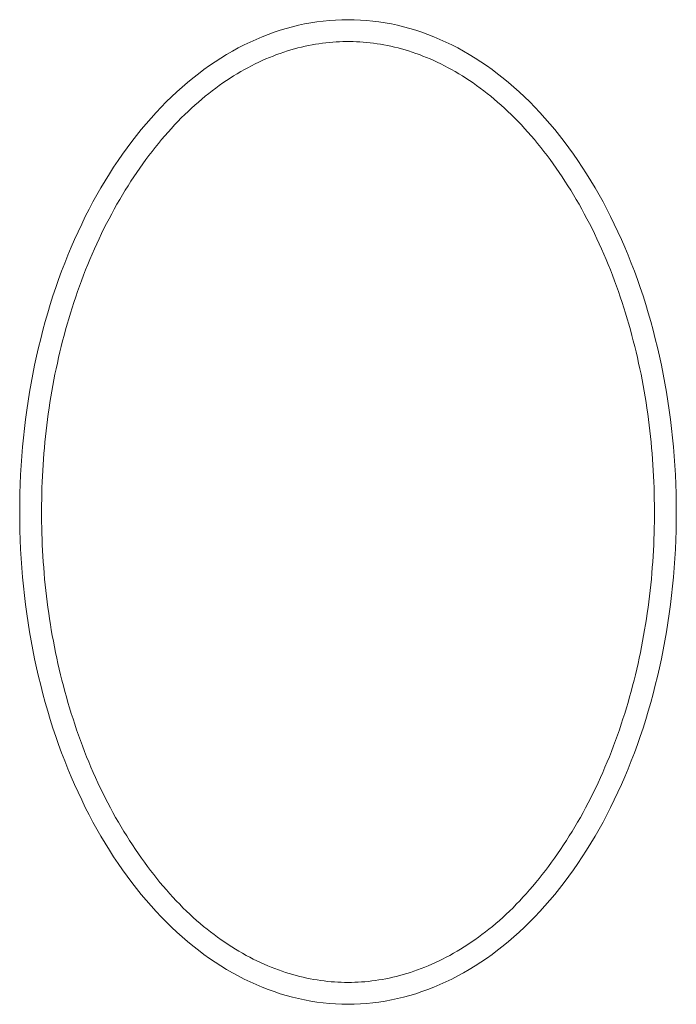
# Model space of a CAD drawing. Units: inches. Extents: x 963 to 2075, y 289 to 2657.
# Tile 52 of 98: x 1538 to 1555, y 1765 to 1790. Entities that reach past the tile are written whole.
import ezdxf

# ---------------------------------------------------------------- set-up
doc = ezdxf.new("R2010")
doc.units = ezdxf.units.IN
doc.layers.add('A-FURN', color=8, linetype='Continuous', lineweight=18)

# ---------------------------------------------------------------- blocks, each defined once
blk = doc.blocks.new('TABLE-OVAL')
at = {"ltscale": 0.03}
blk.add_polyline3d([(7.656, -0.197, 0), (7.809, -0.194, 0), (7.963, -0.188, 0), (8.116, -0.177, 0), (8.269, -0.162, 0), (8.422, -0.142, 0), (8.575, -0.118, 0), (8.727, -0.09, 0), (8.879, -0.057, 0), (9.031, -0.021, 0), (9.182, 0.021, 0), (9.332, 0.066, 0), (9.482, 0.116, 0), (9.632, 0.17, 0), (9.78, 0.228, 0), (9.928, 0.29, 0), (10.075, 0.357, 0), (10.221, 0.428, 0), (10.366, 0.503, 0), (10.51, 0.582, 0), (10.653, 0.665, 0), (10.796, 0.752, 0), (10.937, 0.843, 0), (11.076, 0.938, 0), (11.215, 1.037, 0), (11.352, 1.14, 0), (11.488, 1.247, 0), (11.623, 1.358, 0), (11.756, 1.472, 0), (11.888, 1.59, 0), (12.018, 1.712, 0), (12.147, 1.838, 0), (12.274, 1.967, 0), (12.399, 2.1, 0), (12.523, 2.237, 0), (12.645, 2.376, 0), (12.765, 2.52, 0), (12.883, 2.666, 0), (13, 2.817, 0), (13.114, 2.97, 0), (13.227, 3.126, 0), (13.337, 3.286, 0), (13.446, 3.449, 0), (13.552, 3.615, 0), (13.657, 3.784, 0), (13.759, 3.955, 0), (13.859, 4.13, 0), (13.957, 4.308, 0), (14.052, 4.488, 0), (14.145, 4.671, 0), (14.236, 4.856, 0), (14.325, 5.044, 0), (14.411, 5.235, 0), (14.495, 5.428, 0), (14.576, 5.623, 0), (14.655, 5.821, 0), (14.731, 6.021, 0), (14.805, 6.222, 0), (14.877, 6.426, 0), (14.945, 6.632, 0), (15.011, 6.84, 0), (15.075, 7.05, 0), (15.135, 7.261, 0), (15.193, 7.475, 0), (15.249, 7.689, 0), (15.301, 7.906, 0), (15.351, 8.123, 0), (15.399, 8.343, 0), (15.443, 8.563, 0), (15.485, 8.785, 0), (15.523, 9.007, 0), (15.559, 9.231, 0), (15.592, 9.456, 0), (15.623, 9.682, 0), (15.65, 9.908, 0), (15.675, 10.136, 0), (15.697, 10.364, 0), (15.715, 10.592, 0), (15.731, 10.821, 0), (15.744, 11.051, 0), (15.755, 11.28, 0), (15.762, 11.51, 0), (15.766, 11.741, 0), (15.768, 11.971, 0), (15.766, 12.201, 0), (15.762, 12.431, 0), (15.755, 12.661, 0), (15.744, 12.891, 0), (15.731, 13.12, 0), (15.715, 13.349, 0), (15.697, 13.578, 0), (15.675, 13.806, 0), (15.65, 14.033, 0), (15.623, 14.26, 0), (15.592, 14.486, 0), (15.559, 14.71, 0), (15.523, 14.934, 0), (15.485, 15.157, 0), (15.443, 15.379, 0), (15.399, 15.599, 0), (15.351, 15.818, 0), (15.301, 16.036, 0), (15.249, 16.252, 0), (15.193, 16.467, 0), (15.135, 16.68, 0), (15.075, 16.892, 0), (15.011, 17.101, 0), (14.945, 17.309, 0), (14.877, 17.515, 0), (14.805, 17.719, 0), (14.731, 17.921, 0), (14.655, 18.121, 0), (14.576, 18.318, 0), (14.495, 18.514, 0), (14.411, 18.707, 0), (14.325, 18.897, 0), (14.236, 19.085, 0), (14.145, 19.271, 0), (14.052, 19.454, 0), (13.957, 19.634, 0), (13.859, 19.811, 0), (13.759, 19.986, 0), (13.657, 20.158, 0), (13.552, 20.327, 0), (13.446, 20.493, 0), (13.337, 20.656, 0), (13.227, 20.815, 0), (13.114, 20.972, 0), (13, 21.125, 0), (12.883, 21.275, 0), (12.765, 21.422, 0), (12.645, 21.565, 0), (12.523, 21.705, 0), (12.399, 21.842, 0), (12.274, 21.974, 0), (12.147, 22.104, 0), (12.018, 22.229, 0), (11.888, 22.351, 0), (11.756, 22.47, 0), (11.623, 22.584, 0), (11.488, 22.695, 0), (11.352, 22.802, 0), (11.215, 22.905, 0), (11.076, 23.004, 0), (10.937, 23.099, 0), (10.796, 23.19, 0), (10.653, 23.277, 0), (10.51, 23.36, 0), (10.366, 23.439, 0), (10.221, 23.514, 0), (10.075, 23.585, 0), (9.928, 23.651, 0), (9.78, 23.714, 0), (9.632, 23.772, 0), (9.482, 23.826, 0), (9.332, 23.876, 0), (9.182, 23.921, 0), (9.031, 23.962, 0), (8.879, 23.999, 0), (8.727, 24.032, 0), (8.575, 24.06, 0), (8.422, 24.084, 0), (8.269, 24.103, 0), (8.116, 24.119, 0), (7.963, 24.13, 0), (7.809, 24.136, 0), (7.656, 24.138, 0), (7.502, 24.136, 0), (7.349, 24.13, 0), (7.196, 24.119, 0), (7.042, 24.103, 0), (6.89, 24.084, 0), (6.737, 24.06, 0), (6.585, 24.032, 0), (6.433, 23.999, 0), (6.281, 23.962, 0), (6.13, 23.921, 0), (5.979, 23.876, 0), (5.83, 23.826, 0), (5.68, 23.772, 0), (5.532, 23.714, 0), (5.384, 23.651, 0), (5.237, 23.585, 0), (5.091, 23.514, 0), (4.946, 23.439, 0), (4.802, 23.36, 0), (4.658, 23.277, 0), (4.516, 23.19, 0), (4.375, 23.099, 0), (4.236, 23.004, 0), (4.097, 22.905, 0), (3.96, 22.802, 0), (3.824, 22.695, 0), (3.689, 22.584, 0), (3.556, 22.47, 0), (3.424, 22.351, 0), (3.294, 22.229, 0), (3.165, 22.104, 0), (3.038, 21.974, 0), (2.913, 21.842, 0), (2.789, 21.705, 0), (2.667, 21.565, 0), (2.547, 21.422, 0), (2.429, 21.275, 0), (2.312, 21.125, 0), (2.198, 20.972, 0), (2.085, 20.815, 0), (1.975, 20.656, 0), (1.866, 20.493, 0), (1.76, 20.327, 0), (1.655, 20.158, 0), (1.553, 19.986, 0), (1.453, 19.811, 0), (1.355, 19.634, 0), (1.26, 19.454, 0), (1.166, 19.271, 0), (1.076, 19.085, 0), (0.987, 18.897, 0), (0.901, 18.707, 0), (0.817, 18.514, 0), (0.736, 18.318, 0), (0.657, 18.121, 0), (0.58, 17.921, 0), (0.507, 17.719, 0), (0.435, 17.515, 0), (0.367, 17.309, 0), (0.301, 17.101, 0), (0.237, 16.892, 0), (0.177, 16.68, 0), (0.118, 16.467, 0), (0.063, 16.252, 0), (0.01, 16.036, 0), (-0.039, 15.818, 0), (-0.087, 15.599, 0), (-0.131, 15.379, 0), (-0.173, 15.157, 0), (-0.211, 14.934, 0), (-0.247, 14.71, 0), (-0.281, 14.486, 0), (-0.311, 14.26, 0), (-0.338, 14.033, 0), (-0.363, 13.806, 0), (-0.385, 13.578, 0), (-0.403, 13.349, 0), (-0.419, 13.12, 0), (-0.432, 12.891, 0), (-0.443, 12.661, 0), (-0.45, 12.431, 0), (-0.454, 12.201, 0), (-0.456, 11.971, 0), (-0.454, 11.741, 0), (-0.45, 11.51, 0), (-0.443, 11.28, 0), (-0.432, 11.051, 0), (-0.419, 10.821, 0), (-0.403, 10.592, 0), (-0.385, 10.364, 0), (-0.363, 10.136, 0), (-0.338, 9.908, 0), (-0.311, 9.682, 0), (-0.281, 9.456, 0), (-0.247, 9.231, 0), (-0.211, 9.007, 0), (-0.173, 8.785, 0), (-0.131, 8.563, 0), (-0.087, 8.343, 0), (-0.039, 8.123, 0), (0.01, 7.906, 0), (0.063, 7.689, 0), (0.118, 7.475, 0), (0.177, 7.261, 0), (0.237, 7.05, 0), (0.301, 6.84, 0), (0.367, 6.632, 0), (0.435, 6.426, 0), (0.507, 6.222, 0), (0.58, 6.021, 0), (0.657, 5.821, 0), (0.736, 5.623, 0), (0.817, 5.428, 0), (0.901, 5.235, 0), (0.987, 5.044, 0), (1.076, 4.856, 0), (1.166, 4.671, 0), (1.26, 4.488, 0), (1.355, 4.308, 0), (1.453, 4.13, 0), (1.553, 3.955, 0), (1.655, 3.784, 0), (1.76, 3.615, 0), (1.866, 3.449, 0), (1.975, 3.286, 0), (2.085, 3.126, 0), (2.198, 2.97, 0), (2.312, 2.817, 0), (2.429, 2.666, 0), (2.547, 2.52, 0), (2.667, 2.376, 0), (2.789, 2.237, 0), (2.913, 2.1, 0), (3.038, 1.967, 0), (3.165, 1.838, 0), (3.294, 1.712, 0), (3.424, 1.59, 0), (3.556, 1.472, 0), (3.689, 1.358, 0), (3.824, 1.247, 0), (3.96, 1.14, 0), (4.097, 1.037, 0), (4.236, 0.938, 0), (4.375, 0.843, 0), (4.516, 0.752, 0), (4.658, 0.665, 0), (4.802, 0.582, 0), (4.946, 0.503, 0), (5.091, 0.428, 0), (5.237, 0.357, 0), (5.384, 0.29, 0), (5.532, 0.228, 0), (5.68, 0.17, 0), (5.83, 0.116, 0), (5.979, 0.066, 0), (6.13, 0.021, 0), (6.281, -0.021, 0), (6.433, -0.057, 0), (6.585, -0.09, 0), (6.737, -0.118, 0), (6.89, -0.142, 0), (7.042, -0.162, 0), (7.196, -0.177, 0), (7.349, -0.188, 0), (7.502, -0.194, 0), (7.656, -0.197, 0)], dxfattribs=at)
blk.add_polyline3d([(7.656, 0.344, 0), (7.739, 0.345, 0), (7.822, 0.347, 0), (7.906, 0.351, 0), (7.99, 0.356, 0), (8.074, 0.362, 0), (8.159, 0.37, 0), (8.244, 0.38, 0), (8.33, 0.391, 0), (8.415, 0.404, 0), (8.501, 0.418, 0), (8.588, 0.434, 0), (8.674, 0.451, 0), (8.761, 0.47, 0), (8.848, 0.491, 0), (8.935, 0.513, 0), (9.023, 0.538, 0), (9.11, 0.563, 0), (9.198, 0.591, 0), (9.286, 0.62, 0), (9.375, 0.651, 0), (9.463, 0.684, 0), (9.552, 0.719, 0), (9.64, 0.755, 0), (9.729, 0.794, 0), (9.818, 0.834, 0), (9.907, 0.876, 0), (9.995, 0.92, 0), (10.084, 0.966, 0), (10.173, 1.013, 0), (10.262, 1.063, 0), (10.35, 1.114, 0), (10.439, 1.167, 0), (10.527, 1.222, 0), (10.615, 1.279, 0), (10.703, 1.338, 0), (10.791, 1.398, 0), (10.878, 1.461, 0), (10.965, 1.525, 0), (11.052, 1.592, 0), (11.139, 1.66, 0), (11.225, 1.73, 0), (11.311, 1.802, 0), (11.396, 1.876, 0), (11.481, 1.952, 0), (11.565, 2.03, 0), (11.649, 2.109, 0), (11.733, 2.191, 0), (11.815, 2.275, 0), (11.898, 2.361, 0), (11.98, 2.448, 0), (12.061, 2.537, 0), (12.141, 2.629, 0), (12.221, 2.721, 0), (12.301, 2.816, 0), (12.379, 2.912, 0), (12.457, 3.01, 0), (12.535, 3.11, 0), (12.611, 3.211, 0), (12.687, 3.314, 0), (12.762, 3.418, 0), (12.836, 3.524, 0), (12.909, 3.632, 0), (12.982, 3.741, 0), (13.053, 3.851, 0), (13.124, 3.963, 0), (13.194, 4.076, 0), (13.262, 4.191, 0), (13.33, 4.307, 0), (13.397, 4.424, 0), (13.463, 4.543, 0), (13.528, 4.662, 0), (13.591, 4.783, 0), (13.654, 4.906, 0), (13.716, 5.029, 0), (13.776, 5.154, 0), (13.835, 5.279, 0), (13.893, 5.406, 0), (13.95, 5.534, 0), (14.006, 5.663, 0), (14.061, 5.792, 0), (14.114, 5.923, 0), (14.166, 6.055, 0), (14.217, 6.188, 0), (14.266, 6.321, 0), (14.314, 6.455, 0), (14.361, 6.589, 0), (14.406, 6.723, 0), (14.45, 6.858, 0), (14.493, 6.993, 0), (14.535, 7.129, 0), (14.575, 7.265, 0), (14.614, 7.401, 0), (14.652, 7.537, 0), (14.688, 7.674, 0), (14.724, 7.811, 0), (14.758, 7.948, 0), (14.791, 8.086, 0), (14.822, 8.223, 0), (14.852, 8.361, 0), (14.882, 8.5, 0), (14.909, 8.638, 0), (14.936, 8.777, 0), (14.961, 8.916, 0), (14.986, 9.055, 0), (15.009, 9.194, 0), (15.031, 9.334, 0), (15.051, 9.473, 0), (15.071, 9.613, 0), (15.089, 9.753, 0), (15.106, 9.893, 0), (15.122, 10.033, 0), (15.137, 10.174, 0), (15.151, 10.314, 0), (15.163, 10.455, 0), (15.175, 10.596, 0), (15.185, 10.736, 0), (15.194, 10.877, 0), (15.202, 11.018, 0), (15.209, 11.159, 0), (15.215, 11.3, 0), (15.219, 11.441, 0), (15.223, 11.583, 0), (15.225, 11.724, 0), (15.227, 11.865, 0), (15.227, 12.006, 0), (15.226, 12.147, 0), (15.224, 12.288, 0), (15.221, 12.43, 0), (15.217, 12.571, 0), (15.212, 12.712, 0), (15.205, 12.853, 0), (15.198, 12.994, 0), (15.19, 13.135, 0), (15.18, 13.276, 0), (15.169, 13.416, 0), (15.157, 13.557, 0), (15.144, 13.698, 0), (15.13, 13.838, 0), (15.114, 13.978, 0), (15.098, 14.119, 0), (15.08, 14.259, 0), (15.061, 14.399, 0), (15.041, 14.538, 0), (15.02, 14.678, 0), (14.997, 14.817, 0), (14.974, 14.956, 0), (14.949, 15.095, 0), (14.923, 15.234, 0), (14.896, 15.373, 0), (14.867, 15.511, 0), (14.837, 15.649, 0), (14.806, 15.787, 0), (14.774, 15.925, 0), (14.741, 16.062, 0), (14.706, 16.199, 0), (14.67, 16.336, 0), (14.633, 16.473, 0), (14.595, 16.609, 0), (14.555, 16.745, 0), (14.514, 16.881, 0), (14.472, 17.016, 0), (14.428, 17.151, 0), (14.384, 17.286, 0), (14.338, 17.42, 0), (14.29, 17.554, 0), (14.241, 17.687, 0), (14.191, 17.821, 0), (14.14, 17.953, 0), (14.087, 18.084, 0), (14.034, 18.214, 0), (13.978, 18.344, 0), (13.922, 18.472, 0), (13.865, 18.599, 0), (13.806, 18.725, 0), (13.746, 18.85, 0), (13.685, 18.974, 0), (13.623, 19.097, 0), (13.56, 19.219, 0), (13.495, 19.339, 0), (13.43, 19.458, 0), (13.364, 19.576, 0), (13.296, 19.693, 0), (13.228, 19.808, 0), (13.159, 19.922, 0), (13.089, 20.035, 0), (13.017, 20.146, 0), (12.945, 20.255, 0), (12.873, 20.364, 0), (12.799, 20.47, 0), (12.724, 20.576, 0), (12.649, 20.679, 0), (12.573, 20.781, 0), (12.496, 20.882, 0), (12.418, 20.981, 0), (12.34, 21.078, 0), (12.261, 21.173, 0), (12.182, 21.267, 0), (12.101, 21.359, 0), (12.02, 21.449, 0), (11.939, 21.537, 0), (11.857, 21.624, 0), (11.774, 21.709, 0), (11.691, 21.791, 0), (11.607, 21.872, 0), (11.523, 21.951, 0), (11.438, 22.028, 0), (11.353, 22.103, 0), (11.268, 22.176, 0), (11.182, 22.247, 0), (11.095, 22.316, 0), (11.009, 22.383, 0), (10.922, 22.449, 0), (10.835, 22.512, 0), (10.747, 22.574, 0), (10.659, 22.633, 0), (10.571, 22.691, 0), (10.483, 22.747, 0), (10.395, 22.801, 0), (10.306, 22.854, 0), (10.217, 22.904, 0), (10.129, 22.952, 0), (10.04, 22.999, 0), (9.951, 23.044, 0), (9.862, 23.087, 0), (9.773, 23.128, 0), (9.685, 23.167, 0), (9.596, 23.205, 0), (9.507, 23.24, 0), (9.419, 23.274, 0), (9.331, 23.306, 0), (9.242, 23.336, 0), (9.154, 23.365, 0), (9.067, 23.391, 0), (8.979, 23.416, 0), (8.892, 23.44, 0), (8.804, 23.461, 0), (8.718, 23.481, 0), (8.631, 23.499, 0), (8.544, 23.516, 0), (8.458, 23.531, 0), (8.373, 23.545, 0), (8.287, 23.557, 0), (8.202, 23.567, 0), (8.117, 23.576, 0), (8.032, 23.583, 0), (7.948, 23.589, 0), (7.864, 23.593, 0), (7.781, 23.596, 0), (7.697, 23.597, 0), (7.615, 23.597, 0), (7.531, 23.596, 0), (7.448, 23.593, 0), (7.364, 23.589, 0), (7.28, 23.583, 0), (7.195, 23.576, 0), (7.11, 23.567, 0), (7.025, 23.557, 0), (6.939, 23.545, 0), (6.854, 23.531, 0), (6.767, 23.516, 0), (6.681, 23.499, 0), (6.594, 23.481, 0), (6.507, 23.461, 0), (6.42, 23.44, 0), (6.333, 23.416, 0), (6.245, 23.391, 0), (6.158, 23.365, 0), (6.07, 23.336, 0), (5.981, 23.306, 0), (5.893, 23.274, 0), (5.805, 23.24, 0), (5.716, 23.205, 0), (5.627, 23.167, 0), (5.539, 23.128, 0), (5.45, 23.087, 0), (5.361, 23.044, 0), (5.272, 22.999, 0), (5.183, 22.952, 0), (5.095, 22.904, 0), (5.006, 22.854, 0), (4.917, 22.801, 0), (4.829, 22.747, 0), (4.741, 22.691, 0), (4.653, 22.633, 0), (4.565, 22.574, 0), (4.477, 22.512, 0), (4.39, 22.449, 0), (4.303, 22.383, 0), (4.216, 22.316, 0), (4.13, 22.247, 0), (4.044, 22.176, 0), (3.959, 22.103, 0), (3.874, 22.028, 0), (3.789, 21.951, 0), (3.705, 21.872, 0), (3.621, 21.791, 0), (3.538, 21.709, 0), (3.455, 21.624, 0), (3.373, 21.537, 0), (3.292, 21.449, 0), (3.211, 21.359, 0), (3.13, 21.267, 0), (3.051, 21.173, 0), (2.972, 21.078, 0), (2.893, 20.981, 0), (2.816, 20.882, 0), (2.739, 20.781, 0), (2.663, 20.679, 0), (2.588, 20.576, 0), (2.513, 20.47, 0), (2.439, 20.364, 0), (2.366, 20.255, 0), (2.294, 20.146, 0), (2.223, 20.035, 0), (2.153, 19.922, 0), (2.084, 19.808, 0), (2.016, 19.693, 0), (1.948, 19.576, 0), (1.882, 19.458, 0), (1.817, 19.339, 0), (1.752, 19.219, 0), (1.689, 19.097, 0), (1.627, 18.974, 0), (1.566, 18.85, 0), (1.506, 18.725, 0), (1.447, 18.599, 0), (1.39, 18.472, 0), (1.334, 18.344, 0), (1.278, 18.214, 0), (1.225, 18.084, 0), (1.172, 17.953, 0), (1.121, 17.821, 0), (1.071, 17.687, 0), (1.022, 17.554, 0), (0.974, 17.42, 0), (0.928, 17.286, 0), (0.884, 17.151, 0), (0.84, 17.016, 0), (0.798, 16.881, 0), (0.757, 16.745, 0), (0.717, 16.609, 0), (0.679, 16.473, 0), (0.642, 16.336, 0), (0.606, 16.199, 0), (0.571, 16.062, 0), (0.538, 15.925, 0), (0.505, 15.787, 0), (0.475, 15.649, 0), (0.445, 15.511, 0), (0.416, 15.373, 0), (0.389, 15.234, 0), (0.363, 15.095, 0), (0.338, 14.956, 0), (0.315, 14.817, 0), (0.292, 14.678, 0), (0.271, 14.538, 0), (0.251, 14.399, 0), (0.232, 14.259, 0), (0.214, 14.119, 0), (0.198, 13.978, 0), (0.182, 13.838, 0), (0.168, 13.698, 0), (0.155, 13.557, 0), (0.143, 13.416, 0), (0.132, 13.276, 0), (0.122, 13.135, 0), (0.114, 12.994, 0), (0.106, 12.853, 0), (0.1, 12.712, 0), (0.095, 12.571, 0), (0.091, 12.43, 0), (0.088, 12.288, 0), (0.086, 12.147, 0), (0.085, 12.006, 0), (0.085, 11.865, 0), (0.087, 11.724, 0), (0.089, 11.583, 0), (0.093, 11.441, 0), (0.097, 11.3, 0), (0.103, 11.159, 0), (0.11, 11.018, 0), (0.118, 10.877, 0), (0.127, 10.736, 0), (0.137, 10.596, 0), (0.149, 10.455, 0), (0.161, 10.314, 0), (0.175, 10.174, 0), (0.19, 10.033, 0), (0.206, 9.893, 0), (0.223, 9.753, 0), (0.241, 9.613, 0), (0.261, 9.473, 0), (0.281, 9.334, 0), (0.303, 9.194, 0), (0.326, 9.055, 0), (0.35, 8.916, 0), (0.376, 8.777, 0), (0.403, 8.638, 0), (0.43, 8.5, 0), (0.46, 8.361, 0), (0.49, 8.223, 0), (0.521, 8.086, 0), (0.554, 7.948, 0), (0.588, 7.811, 0), (0.623, 7.674, 0), (0.66, 7.537, 0), (0.698, 7.401, 0), (0.737, 7.265, 0), (0.777, 7.129, 0), (0.819, 6.993, 0), (0.862, 6.858, 0), (0.906, 6.723, 0), (0.951, 6.589, 0), (0.998, 6.455, 0), (1.046, 6.321, 0), (1.095, 6.188, 0), (1.146, 6.055, 0), (1.198, 5.923, 0), (1.251, 5.792, 0), (1.306, 5.663, 0), (1.362, 5.534, 0), (1.418, 5.406, 0), (1.477, 5.279, 0), (1.536, 5.154, 0), (1.596, 5.029, 0), (1.658, 4.906, 0), (1.721, 4.783, 0), (1.784, 4.662, 0), (1.849, 4.543, 0), (1.915, 4.424, 0), (1.982, 4.307, 0), (2.05, 4.191, 0), (2.118, 4.076, 0), (2.188, 3.963, 0), (2.259, 3.851, 0), (2.33, 3.741, 0), (2.403, 3.632, 0), (2.476, 3.524, 0), (2.55, 3.418, 0), (2.625, 3.314, 0), (2.701, 3.211, 0), (2.777, 3.11, 0), (2.855, 3.01, 0), (2.933, 2.912, 0), (3.011, 2.816, 0), (3.09, 2.721, 0), (3.17, 2.629, 0), (3.251, 2.537, 0), (3.332, 2.448, 0), (3.414, 2.361, 0), (3.497, 2.275, 0), (3.579, 2.191, 0), (3.663, 2.109, 0), (3.747, 2.03, 0), (3.831, 1.952, 0), (3.916, 1.876, 0), (4.001, 1.802, 0), (4.087, 1.73, 0), (4.173, 1.66, 0), (4.26, 1.592, 0), (4.347, 1.525, 0), (4.434, 1.461, 0), (4.521, 1.398, 0), (4.609, 1.338, 0), (4.697, 1.279, 0), (4.785, 1.222, 0), (4.873, 1.167, 0), (4.962, 1.114, 0), (5.05, 1.063, 0), (5.139, 1.013, 0), (5.228, 0.966, 0), (5.316, 0.92, 0), (5.405, 0.876, 0), (5.494, 0.834, 0), (5.583, 0.794, 0), (5.672, 0.755, 0), (5.76, 0.719, 0), (5.849, 0.684, 0), (5.937, 0.651, 0), (6.026, 0.62, 0), (6.114, 0.591, 0), (6.201, 0.563, 0), (6.289, 0.538, 0), (6.377, 0.513, 0), (6.464, 0.491, 0), (6.551, 0.47, 0), (6.638, 0.451, 0), (6.724, 0.434, 0), (6.811, 0.418, 0), (6.897, 0.404, 0), (6.982, 0.391, 0), (7.068, 0.38, 0), (7.153, 0.37, 0), (7.237, 0.362, 0), (7.322, 0.356, 0), (7.406, 0.351, 0), (7.49, 0.347, 0), (7.573, 0.345, 0), (7.656, 0.344, 0)])

msp = doc.modelspace()

# ---------------------------------------------------------------- block references
at = {"layer": 'A-FURN'}
msp.add_blockref('TABLE-OVAL', (1538.937, 1765.591), dxfattribs=at)

doc.saveas('drawing.dxf')
